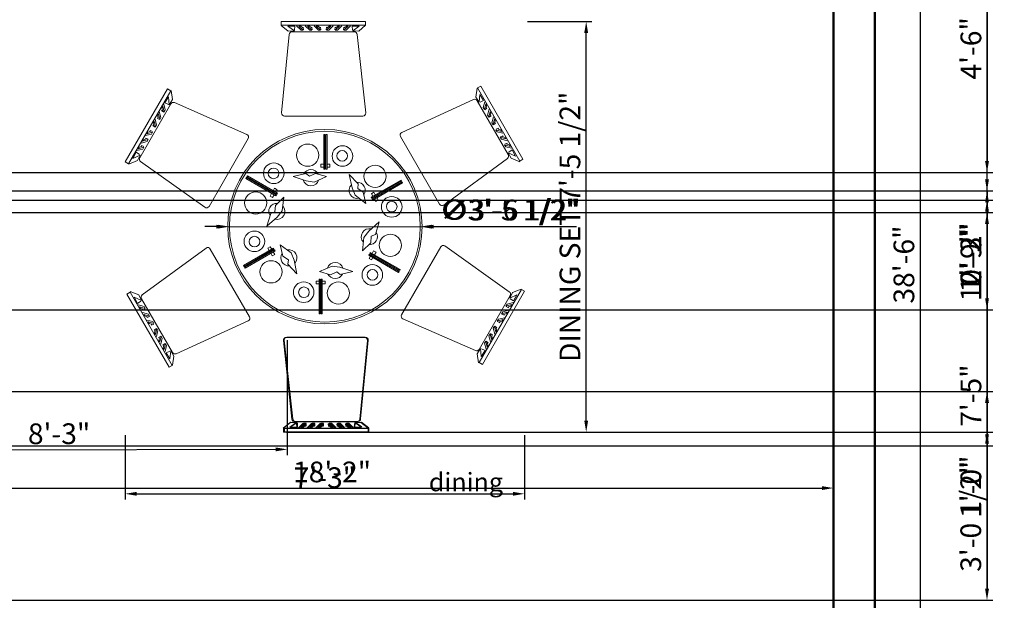
# Model space of a CAD drawing. Units: inches. Extents: x 1253 to 1645, y 2180 to 2698.
# Tile 4 of 5: x 1431 to 1645, y 2363 to 2490. Entities that reach past the tile are written whole.
import ezdxf

# ---------------------------------------------------------------- set-up
doc = ezdxf.new("R2010")
doc.units = ezdxf.units.IN
for name, color, linetype, lineweight in [('A-ANNO-DIMS', 2, 'Continuous', 18), ('A-AREA-IDEN', 7, 'Continuous', 25), ('A-FURN', 8, 'Continuous', 18), ('wall', 7, 'Continuous', 50)]:
    doc.layers.add(name, color=color, linetype=linetype, lineweight=lineweight)
doc.styles.get("Standard").update_dxf_attribs({"font": 'arial.ttf'})
doc.dimstyles.new('ISO-25', dxfattribs={"dimtxt": 4.5, "dimasz": 2.5, "dimexe": 1.25, "dimexo": 0.625, "dimtad": 1, "dimdec": 1, "dimlunit": 3, "dimtxsty": 'Standard', "dimcen": 4.5, "dimadec": 0, "dimazin": 0, "dimtfac": 1, "dimtdec": 1, "dimtmove": 0, "dimatfit": 3, "dimfxl": 1, "dimarcsym": 0})

# ---------------------------------------------------------------- blocks, each defined once
blk = doc.blocks.new('A$C45501D90')
for p, q in [((-242.2, 1133.5), (224, 1133.5)), ((-242.2, 1112.8), (-242.2, 1133.5)), ((224, 1112.8), (-242.2, 1112.8)), ((-242.2, 1111.2), (-202.3, 1079.2)), ((-203.9, 1106.4), (-165.6, 1108)), ((-168.8, 1080.8), (-203.9, 1106.4)), ((-165.6, 1108), (-167.2, 1085.6)), ((-156, 1109.6), (-132, 1085.6)), ((-119.3, 1085.6), (-143.2, 1108)), ((-143.2, 1108), (-133.6, 1108)), ((-133.6, 1108), (-122.5, 1098.4)), ((-122.5, 1098.4), (-119.3, 1101.6)), ((-119.3, 1101.6), (-117.7, 1087.2)), ((-108.1, 1109.6), (-84.1, 1085.6)), ((-71.4, 1085.6), (-95.3, 1108)), ((-95.3, 1108), (-85.7, 1108)), ((-85.7, 1108), (-74.6, 1098.4)), ((-74.6, 1098.4), (-71.4, 1101.6)), ((-71.4, 1101.6), (-69.8, 1087.2)), ((-60.2, 1109.6), (-36.2, 1085.6)), ((-23.5, 1085.6), (-47.4, 1108)), ((-47.4, 1108), (-37.8, 1108)), ((-37.8, 1108), (-26.7, 1098.4)), ((-26.7, 1098.4), (-23.5, 1101.6)), ((-23.5, 1101.6), (-21.9, 1087.2)), ((8.5, 1101.6), (6.9, 1087.2)), ((8.5, 1085.6), (32.4, 1108)), ((11.6, 1098.4), (8.5, 1101.6)), ((22.8, 1108), (11.6, 1098.4)), ((45.2, 1109.6), (21.2, 1085.6)), ((32.4, 1108), (22.8, 1108)), ((56.3, 1101.6), (54.8, 1087.2)), ((56.3, 1085.6), (80.3, 1108)), ((59.5, 1098.4), (56.3, 1101.6)), ((70.7, 1108), (59.5, 1098.4)), ((93.1, 1109.6), (69.1, 1085.6)), ((80.3, 1108), (70.7, 1108)), ((104.2, 1101.6), (102.6, 1087.2)), ((104.2, 1085.6), (128.2, 1108)), ((107.4, 1098.4), (104.2, 1101.6)), ((118.6, 1108), (107.4, 1098.4)), ((141, 1109.6), (117, 1085.6)), ((128.2, 1108), (118.6, 1108)), ((188.9, 1106.4), (150.5, 1108)), ((150.5, 1108), (152.1, 1085.6)), ((153.7, 1080.8), (188.9, 1106.4)), ((224, 1112.8), (187.3, 1079.2)), ((224, 1133.5), (224, 1112.8)), ((-197.3, 1061.6), (-238.9, 627.6)), ((-202.3, 1079.2), (-168.8, 1080.8)), ((161.8, 1076.1), (-181.4, 1076.1)), ((-132, 1085.6), (-119.3, 1085.6)), ((-84.1, 1085.6), (-71.4, 1085.6)), ((-36.2, 1085.6), (-23.5, 1085.6)), ((21.2, 1085.6), (8.5, 1085.6)), ((69.1, 1085.6), (56.3, 1085.6)), ((117, 1085.6), (104.2, 1085.6)), ((187.3, 1079.2), (153.7, 1080.8)), ((225.2, 627.8), (177.6, 1061.8)), ((841.2, 765.3), (833.5, 714.8)), ((842.6, 766.1), (860.5, 776.5)), ((1075.7, 362.4), (842.6, 766.1)), ((860.5, 776.5), (1093.6, 372.8)), ((-1102.7, 357), (-869.7, 760.7)), ((-851.7, 750.4), (-1084.8, 346.6)), ((-863.7, 716.7), (-884.3, 684.4)), ((-869.7, 760.7), (-851.7, 750.4)), ((-859.2, 673.6), (-863.7, 716.7)), ((-848.7, 752.3), (-841, 701.8)), ((833.5, 714.8), (851.7, 686.6)), ((851.7, 686.6), (856.2, 729.8)), ((856.2, 729.8), (876.7, 697.4)), ((-851, 678.1), (-1022.6, 380.9)), ((-895.4, 665), (-900.2, 656.7)), ((-900.2, 656.7), (-897.5, 642.2)), ((-888.1, 633.1), (-895.4, 665)), ((-890.4, 676.9), (-881.7, 644.2)), ((-884.3, 684.4), (-864.1, 674.6)), ((-841, 701.8), (-859.2, 673.6)), ((-431.1, 509), (-830.8, 684.8)), ((820.7, 701.7), (424.1, 520.7)), ((1012.8, 397.9), (841.2, 695.1)), ((876.7, 697.4), (856.6, 687.6)), ((882.9, 689.9), (874.2, 657.2)), ((874.2, 657.2), (880.6, 646.1)), ((880.6, 646.1), (887.9, 678)), ((894.4, 654.1), (882.7, 645.5)), ((887.9, 678), (892.7, 669.7)), ((892.7, 669.7), (890, 655.2)), ((890, 655.2), (894.4, 654.1)), ((-921.5, 600.8), (-925.8, 599.6)), ((-925.8, 599.6), (-914.2, 591)), ((-919.4, 623.5), (-924.2, 615.2)), ((-924.2, 615.2), (-921.5, 600.8)), ((-912, 591.6), (-919.4, 623.5)), ((-914.4, 635.4), (-905.6, 602.7)), ((-905.6, 602.7), (-912, 591.6)), ((-897.5, 642.2), (-901.9, 641.1)), ((-901.9, 641.1), (-890.2, 632.5)), ((-881.7, 644.2), (-888.1, 633.1)), ((-223, 610.1), (209.4, 610.1)), ((906.9, 648.4), (898.1, 615.7)), ((898.1, 615.7), (904.5, 604.6)), ((904.5, 604.6), (911.9, 636.5)), ((918.3, 612.6), (906.7, 604)), ((911.9, 636.5), (916.7, 628.2)), ((916.7, 628.2), (914, 613.8)), ((914, 613.8), (918.3, 612.6)), ((930.8, 606.9), (922.1, 574.2)), ((-945.4, 559.3), (-949.8, 558.1)), ((-949.8, 558.1), (-938.1, 549.6)), ((-943.3, 582), (-948.1, 573.8)), ((-948.1, 573.8), (-945.4, 559.3)), ((-936, 550.1), (-943.3, 582)), ((-938.3, 593.9), (-929.6, 561.2)), ((-929.6, 561.2), (-936, 550.1)), ((922.1, 574.2), (928.4, 563.1)), ((928.4, 563.1), (935.8, 595.1)), ((942.3, 571.1), (930.6, 562.6)), ((935.8, 595.1), (940.6, 586.8)), ((940.6, 586.8), (937.9, 572.3)), ((937.9, 572.3), (942.3, 571.1)), ((-991, 502.7), (-958.3, 511.4)), ((-951.9, 522.5), (-983.2, 512.9)), ((-983.2, 512.9), (-978.5, 521.2)), ((-978.5, 521.2), (-964.6, 526.1)), ((-964.6, 526.1), (-965.7, 530.5)), ((-965.7, 530.5), (-952.5, 524.7)), ((-958.3, 511.4), (-951.9, 522.5)), ((-5.6, 508.7, 90.8), (0.4, 508.7, 90.8)), ((-5.6, 317.7, 90.8), (-5.6, 508.7, 90.8)), ((0.4, 508.7, 90.8), (0.4, 317.7, 90.8)), ((5.8, 317.7, 90.8), (5.8, 508.7, 90.8)), ((5.8, 508.7, 90.8), (11.8, 508.7, 90.8)), ((11.8, 508.7, 90.8), (11.8, 317.7, 90.8)), ((416.9, 498.2), (633.1, 123.7)), ((950.8, 524.4), (944.4, 535.5)), ((944.4, 535.5), (975.7, 525.9)), ((958.2, 543.5), (945, 537.7)), ((983.5, 515.7), (950.8, 524.4)), ((957.1, 539.1), (958.2, 543.5)), ((970.9, 534.2), (957.1, 539.1)), ((968.4, 494), (999.7, 484.4)), ((974.7, 483), (968.4, 494)), ((982.2, 502), (968.9, 496.2)), ((975.7, 525.9), (970.9, 534.2)), ((981, 497.6), (982.2, 502)), ((994.9, 492.7), (981, 497.6)), ((999.7, 484.4), (994.9, 492.7)), ((-999.8, 439.5), (-1031.1, 430)), ((-1031.1, 430), (-1026.3, 438.3)), ((-1026.3, 438.3), (-1012.5, 443.1)), ((-1015, 461.2), (-982.3, 469.9)), ((-1012.5, 443.1), (-1013.6, 447.5)), ((-1013.6, 447.5), (-1000.4, 441.7)), ((-975.9, 481), (-1007.2, 471.4)), ((-1007.2, 471.4), (-1002.4, 479.7)), ((-1006.2, 428.5), (-999.8, 439.5)), ((-1002.4, 479.7), (-988.5, 484.6)), ((-988.5, 484.6), (-989.7, 489)), ((-989.7, 489), (-976.5, 483.2)), ((-982.3, 469.9), (-975.9, 481)), ((-639.9, 111.9), (-423.7, 486.4)), ((1007.4, 474.2), (974.7, 483)), ((998.7, 441.5), (992.3, 452.5)), ((992.3, 452.5), (1023.6, 443)), ((1006.1, 460.5), (992.9, 454.7)), ((1031.4, 432.7), (998.7, 441.5)), ((1005, 456.2), (1006.1, 460.5)), ((1018.8, 451.3), (1005, 456.2)), ((1023.6, 443), (1018.8, 451.3)), ((-1060.1, 376.6), (-1042.3, 410.6)), ((-1020.4, 394.3), (-1060.1, 376.6)), ((-1042.3, 410.6), (-1023.8, 398.1)), ((-1038.9, 419.7), (-1006.2, 428.5)), ((-1035.8, 364.4), (-1020.4, 394.3)), ((1028.3, 377.5), (1012.9, 407.3)), ((1012.9, 407.3), (1052.6, 389.6)), ((1034.8, 423.6), (1016.3, 411.1)), ((1052.6, 389.6), (1034.8, 423.6)), ((-1084.8, 346.6), (-1102.7, 357)), ((-1083.4, 345.8), (-1035.8, 364.4)), ((-1018, 360), (-663, 106.9)), ((-22.3, 329.1, 90.8), (-22.3, 344.6, 90.8)), ((-22.3, 344.6, 90.8), (-5.6, 344.6, 90.8)), ((-5.6, 329.1, 90.8), (-22.3, 329.1, 90.8)), ((0.4, 344.6, 90.8), (5.8, 344.6, 90.8)), ((5.8, 329.1, 90.8), (0.4, 329.1, 90.8)), ((11.8, 344.6, 90.8), (27.3, 344.6, 90.8)), ((27.3, 329.1, 90.8), (11.8, 329.1, 90.8)), ((27.3, 344.6, 90.8), (27.3, 329.1, 90.8)), ((656.3, 118.9), (1008.4, 377.1)), ((1075.9, 358.8), (1028.3, 377.5)), ((1093.6, 372.8), (1075.7, 362.4)), ((-430.6, 275.2, 90.8), (-427.6, 280.3, 90.8)), ((-265.2, 179.7, 90.8), (-430.6, 275.2, 90.8)), ((-427.6, 280.3, 90.8), (-262.3, 184.9, 90.8)), ((-175.3, 276.1, 90.8), (-104.8, 293.2, 90.8)), ((-103.3, 252.4, 90.8), (-175.3, 276.1, 90.8)), ((-104.8, 293.2, 90.8), (-85.5, 278.4, 90.8)), ((-85.5, 278.4, 90.8), (-52.1, 293.9, 90.8)), ((9.5, 276.1, 90.8), (-59.5, 246.5, 90.8)), ((-52.1, 293.9, 90.8), (9.5, 276.1, 90.8)), ((0.4, 317.7, 90.8), (-5.6, 317.7, 90.8)), ((11.8, 317.7, 90.8), (5.8, 317.7, 90.8)), ((134.3, 288, 90.8), (184.3, 235.5, 90.8)), ((149.7, 213.9, 90.8), (134.3, 288, 90.8)), ((-436.3, 265.3, 90.8), (-433.3, 270.5, 90.8)), ((-270.9, 169.9, 90.8), (-436.3, 265.3, 90.8)), ((-433.3, 270.5, 90.8), (-267.9, 175, 90.8)), ((-59.5, 246.5, 90.8), (-103.3, 252.4, 90.8)), ((184.3, 235.5, 90.8), (181.1, 211.4, 90.8)), ((255.2, 161.9, 90.8), (420.6, 257.3, 90.8)), ((423.5, 252.2, 90.8), (258.2, 156.7, 90.8)), ((260.9, 152, 90.8), (426.2, 247.5, 90.8)), ((429.2, 242.3, 90.8), (263.8, 146.9, 90.8)), ((420.6, 257.3, 90.8), (423.5, 252.2, 90.8)), ((426.2, 247.5, 90.8), (429.2, 242.3, 90.8)), ((-302.5, 168.8, 90.8), (-294.2, 183.3, 90.8)), ((-289.1, 161.1, 90.8), (-302.5, 168.8, 90.8)), ((-291.2, 188.5, 90.8), (-288.5, 193.1, 90.8)), ((-280.7, 175.5, 90.8), (-289.1, 161.1, 90.8)), ((-285.5, 198.3, 90.8), (-277.8, 211.7, 90.8)), ((-277.8, 211.7, 90.8), (-264.3, 204, 90.8)), ((-275.1, 185.4, 90.8), (-277.8, 180.7, 90.8)), ((-264.3, 204, 90.8), (-272.1, 190.5, 90.8)), ((-267.9, 175, 90.8), (-270.9, 169.9, 90.8)), ((-262.3, 184.9, 90.8), (-265.2, 179.7, 90.8)), ((166.5, 173, 90.8), (149.7, 213.9, 90.8)), ((226.7, 128.1, 90.8), (166.5, 173, 90.8)), ((181.1, 211.4, 90.8), (211.3, 190.3, 90.8)), ((211.3, 190.3, 90.8), (226.7, 128.1, 90.8)), ((256.6, 182, 90.8), (270.1, 189.8, 90.8)), ((265, 167.5, 90.8), (256.6, 182, 90.8)), ((270.1, 189.8, 90.8), (278.4, 175.3, 90.8)), ((281.4, 170.1, 90.8), (284.1, 165.5, 90.8)), ((-276.8, 80.9, 90.8), (-273.6, 117.6, 90.8)), ((-273.6, 117.6, 90.8), (-227.4, 162.1, 90.8)), ((-227.4, 162.1, 90.8), (-236.2, 87.5, 90.8)), ((258.2, 156.7, 90.8), (255.2, 161.9, 90.8)), ((263.8, 146.9, 90.8), (260.9, 152, 90.8)), ((270.7, 157.7, 90.8), (268, 162.4, 90.8)), ((281.4, 139.1, 90.8), (273.7, 152.5, 90.8)), ((294.9, 146.8, 90.8), (281.4, 139.1, 90.8)), ((287.1, 160.3, 90.8), (294.9, 146.8, 90.8)), ((-319.8, 2.1, 90.8), (-299.3, 71.7, 90.8)), ((-299.3, 71.7, 90.8), (-276.8, 80.9, 90.8)), ((-236.2, 87.5, 90.8), (-263.2, 52.5, 90.8)), ((-263.2, 52.5, 90.8), (-319.8, 2.1, 90.8)), ((242.9, -24.6, 90.8), (299.4, 25.9, 90.8)), ((299.4, 25.9, 90.8), (278.9, -43.7, 90.8)), ((215.8, -59.5, 90.8), (242.9, -24.6, 90.8)), ((256.4, -53, 90.8), (253.2, -89.7, 90.8)), ((278.9, -43.7, 90.8), (256.4, -53, 90.8)), ((-247, -100.1, 90.8), (-186.8, -145, 90.8)), ((-231.7, -162.3, 90.8), (-247, -100.1, 90.8)), ((207, -134.1, 90.8), (215.8, -59.5, 90.8)), ((253.2, -89.7, 90.8), (207, -134.1, 90.8)), ((1018, -360), (663, -106.9)), ((-656.3, -118.9), (-1008.4, -377.1)), ((-416.9, -498.2), (-633.1, -123.7)), ((-449.6, -214.4, 90.8), (-284.2, -118.9, 90.8)), ((-281.2, -124.1, 90.8), (-446.6, -219.5, 90.8)), ((-443.9, -224.2, 90.8), (-278.5, -128.7, 90.8)), ((-275.5, -133.9, 90.8), (-440.9, -229.4, 90.8)), ((-315.2, -118.9, 90.8), (-301.8, -111.1, 90.8)), ((-307.5, -132.3, 90.8), (-315.2, -118.9, 90.8)), ((-301.8, -142.1, 90.8), (-304.5, -137.5, 90.8)), ((-301.8, -111.1, 90.8), (-294, -124.6, 90.8)), ((-290.4, -161.8, 90.8), (-298.8, -147.3, 90.8)), ((-291, -129.7, 90.8), (-288.3, -134.4, 90.8)), ((-277, -154, 90.8), (-290.4, -161.8, 90.8)), ((-285.4, -139.5, 90.8), (-277, -154, 90.8)), ((-284.2, -118.9, 90.8), (-281.2, -124.1, 90.8)), ((-278.5, -128.7, 90.8), (-275.5, -133.9, 90.8)), ((-201.5, -183.4, 90.8), (-231.7, -162.3, 90.8)), ((-186.8, -145, 90.8), (-170.1, -185.9, 90.8)), ((241.9, -156.9, 90.8), (244.9, -151.7, 90.8)), ((407.3, -252.4, 90.8), (241.9, -156.9, 90.8)), ((244, -176, 90.8), (251.7, -162.5, 90.8)), ((244.9, -151.7, 90.8), (410.3, -247.2, 90.8)), ((247.6, -147.1, 90.8), (250.6, -141.9, 90.8)), ((413, -242.5, 90.8), (247.6, -147.1, 90.8)), ((250.6, -141.9, 90.8), (415.9, -237.4, 90.8)), ((254.7, -157.4, 90.8), (257.4, -152.7, 90.8)), ((260.4, -147.6, 90.8), (268.7, -133.1, 90.8)), ((270.8, -160.5, 90.8), (268.1, -165.1, 90.8)), ((268.7, -133.1, 90.8), (282.2, -140.8, 90.8)), ((282.2, -140.8, 90.8), (273.8, -155.3, 90.8)), ((639.9, -111.9), (423.7, -486.4)), ((-446.6, -219.5, 90.8), (-449.6, -214.4, 90.8)), ((-204.7, -207.6, 90.8), (-201.5, -183.4, 90.8)), ((-154.7, -260.1, 90.8), (-204.7, -207.6, 90.8)), ((-170.1, -185.9, 90.8), (-154.7, -260.1, 90.8)), ((257.4, -183.7, 90.8), (244, -176, 90.8)), ((265.2, -170.3, 90.8), (257.4, -183.7, 90.8)), ((-440.9, -229.4, 90.8), (-443.9, -224.2, 90.8)), ((-29.8, -248.2, 90.8), (39.2, -218.5, 90.8)), ((31.8, -266, 90.8), (-29.8, -248.2, 90.8)), ((65.2, -250.4, 90.8), (31.8, -266, 90.8)), ((39.2, -218.5, 90.8), (83, -224.4, 90.8)), ((84.4, -265.2, 90.8), (65.2, -250.4, 90.8)), ((83, -224.4, 90.8), (154.9, -248.2, 90.8)), ((154.9, -248.2, 90.8), (84.4, -265.2, 90.8)), ((410.3, -247.2, 90.8), (407.3, -252.4, 90.8)), ((415.9, -237.4, 90.8), (413, -242.5, 90.8)), ((-47.6, -316.6, 90.8), (-47.6, -301.1, 90.8)), ((-47.6, -301.1, 90.8), (-32.1, -301.1, 90.8)), ((-32.1, -316.6, 90.8), (-47.6, -316.6, 90.8)), ((-32.1, -480.7, 90.8), (-32.1, -289.8, 90.8)), ((-32.1, -289.8, 90.8), (-26.1, -289.8, 90.8)), ((-26.1, -289.8, 90.8), (-26.1, -480.7, 90.8)), ((-26.1, -301.1, 90.8), (-20.8, -301.1, 90.8)), ((-20.8, -316.6, 90.8), (-26.1, -316.6, 90.8)), ((-20.8, -480.7, 90.8), (-20.8, -289.8, 90.8)), ((-20.8, -289.8, 90.8), (-14.8, -289.8, 90.8)), ((-14.8, -289.8, 90.8), (-14.8, -480.7, 90.8)), ((-14.8, -301.1, 90.8), (1.9, -301.1, 90.8)), ((1.9, -316.6, 90.8), (-14.8, -316.6, 90.8)), ((1.9, -301.1, 90.8), (1.9, -316.6, 90.8)), ((-1093.6, -372.8), (-1075.7, -362.4)), ((-860.5, -776.5), (-1093.6, -372.8)), ((-1075.9, -358.8), (-1028.3, -377.5)), ((-1075.7, -362.4), (-842.6, -766.1)), ((-1028.3, -377.5), (-1012.9, -407.3)), ((851.7, -750.4), (1084.8, -346.6)), ((1102.7, -357), (869.7, -760.7)), ((1035.8, -364.4), (1020.4, -394.3)), ((1020.4, -394.3), (1060.1, -376.6)), ((1083.4, -345.8), (1035.8, -364.4)), ((1060.1, -376.6), (1042.3, -410.6)), ((1084.8, -346.6), (1102.7, -357)), ((-1052.6, -389.6), (-1034.8, -423.6)), ((-1012.9, -407.3), (-1052.6, -389.6)), ((-1034.8, -423.6), (-1016.3, -411.1)), ((-1031.4, -432.7), (-998.7, -441.5)), ((-1012.8, -397.9), (-841.2, -695.1)), ((851, -678.1), (1022.6, -380.9)), ((1006.2, -428.5), (999.8, -439.5)), ((999.8, -439.5), (1031.1, -430)), ((1038.9, -419.7), (1006.2, -428.5)), ((1042.3, -410.6), (1023.8, -398.1)), ((1031.1, -430), (1026.3, -438.3)), ((-1023.6, -443), (-1018.8, -451.3)), ((-992.3, -452.5), (-1023.6, -443)), ((-1018.8, -451.3), (-1005, -456.2)), ((-1007.4, -474.2), (-974.7, -483)), ((-1006.1, -460.5), (-992.9, -454.7)), ((-1005, -456.2), (-1006.1, -460.5)), ((-968.4, -494), (-999.7, -484.4)), ((-999.7, -484.4), (-994.9, -492.7)), ((-998.7, -441.5), (-992.3, -452.5)), ((-974.7, -483), (-968.4, -494)), ((-26.1, -480.7, 90.8), (-32.1, -480.7, 90.8)), ((-14.8, -480.7, 90.8), (-20.8, -480.7, 90.8)), ((982.3, -469.9), (975.9, -481)), ((975.9, -481), (1007.2, -471.4)), ((989.7, -489), (976.5, -483.2)), ((1015, -461.2), (982.3, -469.9)), ((1002.4, -479.7), (988.5, -484.6)), ((988.5, -484.6), (989.7, -489)), ((1013.6, -447.5), (1000.4, -441.7)), ((1007.2, -471.4), (1002.4, -479.7)), ((1026.3, -438.3), (1012.5, -443.1)), ((1012.5, -443.1), (1013.6, -447.5)), ((-994.9, -492.7), (-981, -497.6)), ((-983.5, -515.7), (-950.8, -524.4)), ((-982.2, -502), (-968.9, -496.2)), ((-981, -497.6), (-982.2, -502)), ((-944.4, -535.5), (-975.7, -525.9)), ((-975.7, -525.9), (-970.9, -534.2)), ((-970.9, -534.2), (-957.1, -539.1)), ((-958.2, -543.5), (-945, -537.7)), ((-957.1, -539.1), (-958.2, -543.5)), ((-950.8, -524.4), (-944.4, -535.5)), ((-820.7, -701.7), (-424.1, -520.7)), ((431.1, -509), (830.8, -684.8)), ((958.3, -511.4), (951.9, -522.5)), ((951.9, -522.5), (983.2, -512.9)), ((965.7, -530.5), (952.5, -524.7)), ((991, -502.7), (958.3, -511.4)), ((978.5, -521.2), (964.6, -526.1)), ((964.6, -526.1), (965.7, -530.5)), ((983.2, -512.9), (978.5, -521.2)), ((-942.3, -571.1), (-930.6, -562.6)), ((-937.9, -572.3), (-942.3, -571.1)), ((-940.6, -586.8), (-937.9, -572.3)), ((-935.8, -595.1), (-940.6, -586.8)), ((-928.4, -563.1), (-935.8, -595.1)), ((-930.8, -606.9), (-922.1, -574.2)), ((-922.1, -574.2), (-928.4, -563.1)), ((905.6, -602.7), (912, -591.6)), ((912, -591.6), (919.4, -623.5)), ((925.8, -599.6), (914.2, -591)), ((929.6, -561.2), (936, -550.1)), ((938.3, -593.9), (929.6, -561.2)), ((936, -550.1), (943.3, -582)), ((949.8, -558.1), (938.1, -549.6)), ((943.3, -582), (948.1, -573.8)), ((945.4, -559.3), (949.8, -558.1)), ((948.1, -573.8), (945.4, -559.3)), ((-918.3, -612.6), (-906.7, -604)), ((-914, -613.8), (-918.3, -612.6)), ((-916.7, -628.2), (-914, -613.8)), ((-911.9, -636.5), (-916.7, -628.2)), ((-904.5, -604.6), (-911.9, -636.5)), ((-906.9, -648.4), (-898.1, -615.7)), ((-898.1, -615.7), (-904.5, -604.6)), ((-894.4, -654.1), (-882.7, -645.5)), ((-880.6, -646.1), (-887.9, -678)), ((-874.2, -657.2), (-880.6, -646.1)), ((-229.3, -629.3), (-181.8, -1063.3)), ((-225.2, -627.8), (-177.6, -1061.8)), ((218.9, -611.6), (-213.5, -611.6)), ((223, -610.1), (-209.4, -610.1)), ((193.2, -1063.1), (234.8, -629.1)), ((197.3, -1061.6), (238.9, -627.6)), ((881.7, -644.2), (888.1, -633.1)), ((890.4, -676.9), (881.7, -644.2)), ((888.1, -633.1), (895.4, -665)), ((901.9, -641.1), (890.2, -632.5)), ((897.5, -642.2), (901.9, -641.1)), ((900.2, -656.7), (897.5, -642.2)), ((914.4, -635.4), (905.6, -602.7)), ((919.4, -623.5), (924.2, -615.2)), ((921.5, -600.8), (925.8, -599.6)), ((924.2, -615.2), (921.5, -600.8)), ((-890, -655.2), (-894.4, -654.1)), ((-892.7, -669.7), (-890, -655.2)), ((-887.9, -678), (-892.7, -669.7)), ((-882.9, -689.9), (-874.2, -657.2)), ((-876.7, -697.4), (-856.6, -687.6)), ((-856.2, -729.8), (-876.7, -697.4)), ((-851.7, -686.6), (-856.2, -729.8)), ((-833.5, -714.8), (-851.7, -686.6)), ((841, -701.8), (859.2, -673.6)), ((848.7, -752.3), (841, -701.8)), ((859.2, -673.6), (863.7, -716.7)), ((863.7, -716.7), (884.3, -684.4)), ((884.3, -684.4), (864.1, -674.6)), ((895.4, -665), (900.2, -656.7)), ((-841.2, -765.3), (-833.5, -714.8)), ((869.7, -760.7), (851.7, -750.4)), ((-842.6, -766.1), (-860.5, -776.5)), ((-231.3, -1112.7), (-191.4, -1080.8)), ((-227.2, -1111.2), (-187.3, -1079.2)), ((-157.9, -1082.4), (-193, -1107.9)), ((-191.4, -1080.8), (-157.9, -1082.4)), ((-153.7, -1080.8), (-188.9, -1106.4)), ((-187.3, -1079.2), (-153.7, -1080.8)), ((-165.9, -1077.6), (177.3, -1077.6)), ((-161.8, -1076.1), (181.4, -1076.1)), ((-154.7, -1109.5), (-156.3, -1087.1)), ((-150.5, -1108), (-152.1, -1085.6)), ((-145.1, -1111.1), (-121.1, -1087.1)), ((-141, -1109.6), (-117, -1085.6)), ((-108.4, -1087.1), (-132.3, -1109.5)), ((-104.2, -1085.6), (-128.2, -1108)), ((-121.1, -1087.1), (-108.4, -1087.1)), ((-117, -1085.6), (-104.2, -1085.6)), ((-104.2, -1101.6), (-102.6, -1087.2)), ((-97.2, -1111.1), (-73.2, -1087.1)), ((-93.1, -1109.6), (-69.1, -1085.6)), ((-60.5, -1087.1), (-84.4, -1109.5)), ((-56.3, -1085.6), (-80.3, -1108)), ((-73.2, -1087.1), (-60.5, -1087.1)), ((-69.1, -1085.6), (-56.3, -1085.6)), ((-56.3, -1101.6), (-54.8, -1087.2)), ((-49.3, -1111.1), (-25.3, -1087.1)), ((-45.2, -1109.6), (-21.2, -1085.6)), ((-12.6, -1087.1), (-36.5, -1109.5)), ((-8.5, -1085.6), (-32.4, -1108)), ((-25.3, -1087.1), (-12.6, -1087.1)), ((-21.2, -1085.6), (-8.5, -1085.6)), ((-8.5, -1101.6), (-6.9, -1087.2)), ((19.4, -1087.1), (43.3, -1109.5)), ((32.1, -1087.1), (19.4, -1087.1)), ((23.5, -1101.6), (21.9, -1087.2)), ((23.5, -1085.6), (47.4, -1108)), ((36.2, -1085.6), (23.5, -1085.6)), ((56.1, -1111.1), (32.1, -1087.1)), ((60.2, -1109.6), (36.2, -1085.6)), ((67.3, -1087.1), (91.2, -1109.5)), ((80, -1087.1), (67.3, -1087.1)), ((71.4, -1101.6), (69.8, -1087.2)), ((71.4, -1085.6), (95.3, -1108)), ((84.1, -1085.6), (71.4, -1085.6)), ((104, -1111.1), (80, -1087.1)), ((108.1, -1109.6), (84.1, -1085.6)), ((115.1, -1087.1), (139.1, -1109.5)), ((127.9, -1087.1), (115.1, -1087.1)), ((119.3, -1101.6), (117.7, -1087.2)), ((119.3, -1085.6), (143.2, -1108)), ((132, -1085.6), (119.3, -1085.6)), ((151.9, -1111.1), (127.9, -1087.1)), ((156, -1109.6), (132, -1085.6)), ((161.4, -1109.5), (163, -1087.1)), ((198.2, -1080.8), (164.6, -1082.4)), ((164.6, -1082.4), (199.8, -1107.9)), ((165.6, -1108), (167.2, -1085.6)), ((202.3, -1079.2), (168.8, -1080.8)), ((168.8, -1080.8), (203.9, -1106.4)), ((238.1, -1112.7), (198.2, -1080.8)), ((242.2, -1111.2), (202.3, -1079.2)), ((-228.1, -1114.3), (238.1, -1114.3)), ((-228.1, -1135), (-228.1, -1114.3)), ((238.1, -1135), (-228.1, -1135)), ((-224, -1112.8), (242.2, -1112.8)), ((-224, -1133.5), (-224, -1112.8)), ((242.2, -1133.5), (-224, -1133.5)), ((-193, -1107.9), (-154.7, -1109.5)), ((-188.9, -1106.4), (-150.5, -1108)), ((-132.3, -1109.5), (-122.7, -1109.5)), ((-128.2, -1108), (-118.6, -1108)), ((-122.7, -1109.5), (-111.6, -1099.9)), ((-118.6, -1108), (-107.4, -1098.4)), ((-111.6, -1099.9), (-108.4, -1103.1)), ((-108.4, -1103.1), (-106.8, -1088.7)), ((-107.4, -1098.4), (-104.2, -1101.6)), ((-84.4, -1109.5), (-74.8, -1109.5)), ((-80.3, -1108), (-70.7, -1108)), ((-74.8, -1109.5), (-63.7, -1099.9)), ((-70.7, -1108), (-59.5, -1098.4)), ((-63.7, -1099.9), (-60.5, -1103.1)), ((-60.5, -1103.1), (-58.9, -1088.7)), ((-59.5, -1098.4), (-56.3, -1101.6)), ((-36.5, -1109.5), (-26.9, -1109.5)), ((-32.4, -1108), (-22.8, -1108)), ((-26.9, -1109.5), (-15.8, -1099.9)), ((-22.8, -1108), (-11.6, -1098.4)), ((-15.8, -1099.9), (-12.6, -1103.1)), ((-12.6, -1103.1), (-11, -1088.7)), ((-11.6, -1098.4), (-8.5, -1101.6)), ((19.4, -1103.1), (17.8, -1088.7)), ((22.6, -1099.9), (19.4, -1103.1)), ((33.7, -1109.5), (22.6, -1099.9)), ((26.7, -1098.4), (23.5, -1101.6)), ((37.8, -1108), (26.7, -1098.4)), ((43.3, -1109.5), (33.7, -1109.5)), ((47.4, -1108), (37.8, -1108)), ((67.3, -1103.1), (65.7, -1088.7)), ((70.4, -1099.9), (67.3, -1103.1)), ((81.6, -1109.5), (70.4, -1099.9)), ((74.6, -1098.4), (71.4, -1101.6)), ((85.7, -1108), (74.6, -1098.4)), ((91.2, -1109.5), (81.6, -1109.5)), ((95.3, -1108), (85.7, -1108)), ((115.1, -1103.1), (113.6, -1088.7)), ((118.3, -1099.9), (115.1, -1103.1)), ((129.5, -1109.5), (118.3, -1099.9)), ((122.5, -1098.4), (119.3, -1101.6)), ((133.6, -1108), (122.5, -1098.4)), ((139.1, -1109.5), (129.5, -1109.5)), ((143.2, -1108), (133.6, -1108)), ((199.8, -1107.9), (161.4, -1109.5)), ((203.9, -1106.4), (165.6, -1108)), ((238.1, -1114.3), (238.1, -1135)), ((242.2, -1112.8), (242.2, -1133.5))]:
    blk.add_line(p, q)
for centre, radius in [((0, 0), 537), ((0, 0), 527), ((-94.8, 394.7, 90.8), 61.3), ((96.9, 390, 90.8), 56.9), ((95.5, 390.7, 90.8), 29.4), ((-282.3, 294.7, 90.8), 56.9), ((277.2, 277.6, 90.8), 61.3), ((-283.5, 293.9, 90.8), 29.4), ((-382.1, 131.1, 90.8), 61.3), ((369, 109.3, 90.8), 56.9), ((368.9, 110.8, 90.8), 29.4), ((-389.3, -81.3, 90.8), 56.9), ((-389.2, -82.8, 90.8), 29.4), ((361.8, -103.1, 90.8), 61.3), ((-297.5, -249.6, 90.8), 61.3), ((261.9, -266.7, 90.8), 56.9), ((263.2, -265.9, 90.8), 29.4), ((-117.2, -362, 90.8), 56.9), ((74.4, -366.7, 90.8), 61.3), ((-115.9, -362.7, 90.8), 29.4)]:
    blk.add_circle(centre, radius)
for centre, radius, start, end in [((-181.4, 1060.1), 16, 90, 174.5199), ((161.8, 1060.1), 16, 6.2572, 90), ((-837.2, 670.1), 16, 66.2572, 150), ((827.4, 687.1), 16, 30, 114.5199), ((-223, 626.1), 16, 174.5199, 270), ((209.4, 626.1), 16, 270, 6.2572), ((-437.5, 494.4), 16, 330, 66.2572), ((430.7, 506.2), 16, 114.5199, 210), ((-1008.8, 373), 16, 150, 234.5199), ((999, 389.9), 16, 306.2572, 30), ((-77.3, 270.2, 90.8), 44.6, 25.8558, 153.3359), ((-77.3, 270.2, 90.8), 44.6, 195.9338, 342.9389), ((178.1, 200.3, 90.8), 44.6, 135.9338, 282.9389), ((178.1, 200.3, 90.8), 44.6, 325.8558, 93.3359), ((-653.7, 119.9), 16, 234.5199, 330), ((-265.7, 83.9, 90.8), 44.6, 85.8558, 213.3359), ((-265.7, 83.9, 90.8), 44.6, 255.9338, 42.9389), ((646.9, 131.7), 16, 210, 306.2572), ((245.3, -55.9, 90.8), 44.6, 75.9338, 222.9389), ((245.3, -55.9, 90.8), 44.6, 265.8558, 33.3359), ((653.7, -119.9), 16, 54.5199, 150), ((-646.9, -131.7), 16, 30, 126.2572), ((-198.5, -172.3, 90.8), 44.6, 145.8558, 273.3359), ((-198.5, -172.3, 90.8), 44.6, 315.9338, 102.9389), ((57, -242.2, 90.8), 44.6, 15.9338, 162.9389), ((57, -242.2, 90.8), 44.6, 205.8558, 333.3359), ((-999, -389.9), 16, 126.2572, 210), ((1008.8, -373), 16, 330, 54.5199), ((437.5, -494.4), 16, 150, 246.2572), ((-430.7, -506.2), 16, 294.5199, 30), ((-213.5, -627.6), 16, 90, 186.2572), ((-209.4, -626.1), 16, 90, 186.2572), ((218.9, -627.6), 16, 354.5199, 90), ((223, -626.1), 16, 354.5199, 90), ((-827.4, -687.1), 16, 210, 294.5199), ((837.2, -670.1), 16, 246.2572, 330), ((-165.9, -1061.6), 16, 186.2572, 270), ((-161.8, -1060.1), 16, 186.2572, 270), ((177.3, -1061.6), 16, 270, 354.5199), ((181.4, -1060.1), 16, 270, 354.5199)]:
    blk.add_arc(centre, radius, start, end)
blk = doc.blocks.new('*D14')
at = {"layer": 'A-ANNO-DIMS', "color": 0, "lineweight": -2, "transparency": 16777216}
for p, q in [((1617.57, 2667.35), (1628.02, 2667.35)), ((1626.77, 2664.85), (1626.77, 2207.85)), ((1617.57, 2205.35), (1628.02, 2205.35))]:
    blk.add_line(p, q, dxfattribs=at)
at = {"layer": 'A-ANNO-DIMS', "color": 0, "transparency": 16777216}
for points in [[(1626.36, 2664.85), (1627.19, 2664.85), (1626.77, 2667.35)], [(1626.36, 2207.85), (1627.19, 2207.85), (1626.77, 2205.35)]]:
    blk.add_solid(points, dxfattribs=at)
at = {"layer": 'Defpoints', "color": 0, "transparency": 16777216}
for p in [(1616.94, 2667.35), (1616.94, 2205.35), (1626.77, 2205.35)]:
    blk.add_point(p, dxfattribs=at)
at = {"layer": 'A-ANNO-DIMS', "color": 0, "transparency": 16777216, "insert": (1623.85, 2436.35), "char_height": 4.5, "attachment_point": 5, "rotation": 90}
blk.add_mtext('38\'-6"', dxfattribs=at)
blk = doc.blocks.new('*D26')
at = {"layer": 'A-ANNO-DIMS', "color": 0, "lineweight": -2, "transparency": 16777216}
for p, q in [((1541.42, 2489.21), (1555.44, 2489.21)), ((1554.19, 2402.4), (1554.19, 2486.71)), ((1541.42, 2399.9), (1555.44, 2399.9))]:
    blk.add_line(p, q, dxfattribs=at)
at = {"layer": 'A-ANNO-DIMS', "color": 0, "transparency": 16777216}
for points in [[(1553.77, 2486.71), (1554.61, 2486.71), (1554.19, 2489.21)], [(1553.77, 2402.4), (1554.61, 2402.4), (1554.19, 2399.9)]]:
    blk.add_solid(points, dxfattribs=at)
at = {"layer": 'Defpoints', "color": 0, "transparency": 16777216}
for p in [(1540.79, 2489.21), (1554.19, 2489.21), (1540.79, 2399.9)]:
    blk.add_point(p, dxfattribs=at)
at = {"layer": 'A-ANNO-DIMS', "color": 0, "transparency": 16777216, "insert": (1551.24, 2444.56), "char_height": 4.5, "attachment_point": 5, "rotation": 90}
blk.add_mtext('DINING SET 7\'-5 1/2"', dxfattribs=at)
blk = doc.blocks.new('*D27')
at = {"layer": 'A-ANNO-DIMS', "color": 0, "lineweight": -2, "transparency": 16777216}
for p, q in [((1453.96, 2399.27), (1453.96, 2385.25)), ((1540.79, 2399.27), (1540.79, 2385.25)), ((1456.46, 2386.5), (1538.29, 2386.5))]:
    blk.add_line(p, q, dxfattribs=at)
at = {"layer": 'A-ANNO-DIMS', "color": 0, "transparency": 16777216}
for points in [[(1456.46, 2386.92), (1456.46, 2386.09), (1453.96, 2386.5)], [(1538.29, 2386.92), (1538.29, 2386.09), (1540.79, 2386.5)]]:
    blk.add_solid(points, dxfattribs=at)
at = {"layer": 'Defpoints', "color": 0, "transparency": 16777216}
for p in [(1453.96, 2399.9), (1540.79, 2399.9), (1540.79, 2386.5)]:
    blk.add_point(p, dxfattribs=at)
at = {"layer": 'A-ANNO-DIMS', "color": 0, "transparency": 16777216, "insert": (1497.38, 2389.43), "char_height": 4.5, "attachment_point": 5}
blk.add_mtext('7\'-3"', dxfattribs=at)
blk = doc.blocks.new('*D31')
at = {"layer": 'A-ANNO-DIMS', "color": 0, "lineweight": -2, "transparency": 16777216}
for p, q in [((1386.57, 2510.35), (1642.59, 2510.35)), ((1641.34, 2507.85), (1641.34, 2458.85)), ((1386.57, 2456.35), (1642.59, 2456.35))]:
    blk.add_line(p, q, dxfattribs=at)
at = {"layer": 'A-ANNO-DIMS', "color": 0, "transparency": 16777216}
for points in [[(1640.92, 2507.85), (1641.76, 2507.85), (1641.34, 2510.35)], [(1640.92, 2458.85), (1641.76, 2458.85), (1641.34, 2456.35)]]:
    blk.add_solid(points, dxfattribs=at)
at = {"layer": 'Defpoints', "color": 0, "transparency": 16777216}
for p in [(1385.94, 2510.35), (1385.94, 2456.35), (1641.34, 2456.35)]:
    blk.add_point(p, dxfattribs=at)
at = {"layer": 'A-ANNO-DIMS', "color": 0, "transparency": 16777216, "insert": (1638.42, 2483.35), "char_height": 4.5, "attachment_point": 5, "rotation": 90}
blk.add_mtext('4\'-6"', dxfattribs=at)
blk = doc.blocks.new('*D32')
at = {"layer": 'A-ANNO-DIMS', "color": 0, "lineweight": -2, "transparency": 16777216}
for p, q in [((1386.57, 2452.35), (1642.59, 2452.35)), ((1641.34, 2449.85), (1641.34, 2365.85)), ((1386.57, 2363.35), (1642.59, 2363.35))]:
    blk.add_line(p, q, dxfattribs=at)
at = {"layer": 'A-ANNO-DIMS', "color": 0, "transparency": 16777216}
for points in [[(1640.92, 2449.85), (1641.76, 2449.85), (1641.34, 2452.35)], [(1640.92, 2365.85), (1641.76, 2365.85), (1641.34, 2363.35)]]:
    blk.add_solid(points, dxfattribs=at)
at = {"layer": 'Defpoints', "color": 0, "transparency": 16777216}
for p in [(1385.94, 2452.35), (1385.94, 2363.35), (1641.34, 2363.35)]:
    blk.add_point(p, dxfattribs=at)
at = {"layer": 'A-ANNO-DIMS', "color": 0, "transparency": 16777216, "insert": (1638.43, 2407.85), "char_height": 4.5, "attachment_point": 5, "rotation": 90}
blk.add_mtext('7\'-5"', dxfattribs=at)
blk = doc.blocks.new('*D47')
at = {"layer": 'A-ANNO-DIMS', "color": 0, "lineweight": -2, "transparency": 16777216}
for p, q in [((1641.34, 2454.85), (1641.34, 2457.35)), ((1386.57, 2452.35), (1642.59, 2452.35)), ((1641.34, 2452.35), (1641.34, 2450.35)), ((1386.57, 2450.35), (1642.59, 2450.35)), ((1641.34, 2447.85), (1641.34, 2432.13))]:
    blk.add_line(p, q, dxfattribs=at)
at = {"layer": 'A-ANNO-DIMS', "color": 0, "transparency": 16777216}
for points in [[(1640.92, 2454.85), (1641.76, 2454.85), (1641.34, 2452.35)], [(1640.92, 2447.85), (1641.76, 2447.85), (1641.34, 2450.35)]]:
    blk.add_solid(points, dxfattribs=at)
at = {"layer": 'Defpoints', "color": 0, "transparency": 16777216}
for p in [(1385.94, 2452.35), (1385.94, 2450.35), (1641.34, 2450.35)]:
    blk.add_point(p, dxfattribs=at)
at = {"layer": 'A-ANNO-DIMS', "color": 0, "transparency": 16777216, "insert": (1638.42, 2438.74), "char_height": 4.5, "attachment_point": 5, "rotation": 90}
blk.add_mtext('0\'-2"', dxfattribs=at)
blk = doc.blocks.new('*D50')
at = {"layer": 'A-ANNO-DIMS', "color": 0, "lineweight": -2, "transparency": 16777216}
for p, q in [((1363.3, 2408.78), (1642.59, 2408.78)), ((1641.34, 2406.28), (1641.34, 2399.44)), ((1363.3, 2396.94), (1642.59, 2396.94)), ((1641.34, 2396.94), (1641.34, 2381.65))]:
    blk.add_line(p, q, dxfattribs=at)
at = {"layer": 'A-ANNO-DIMS', "color": 0, "transparency": 16777216}
for points in [[(1640.92, 2406.28), (1641.76, 2406.28), (1641.34, 2408.78)], [(1640.92, 2399.44), (1641.76, 2399.44), (1641.34, 2396.94)]]:
    blk.add_solid(points, dxfattribs=at)
at = {"layer": 'Defpoints', "color": 0, "transparency": 16777216}
for p in [(1362.68, 2408.78), (1362.68, 2396.94), (1641.34, 2396.94)]:
    blk.add_point(p, dxfattribs=at)
at = {"layer": 'A-ANNO-DIMS', "color": 0, "transparency": 16777216, "insert": (1638.42, 2388.04), "char_height": 4.5, "attachment_point": 5, "rotation": 90}
blk.add_mtext('1\'-0"', dxfattribs=at)
blk = doc.blocks.new('*D55')
at = {"layer": 'A-ANNO-DIMS', "color": 0, "lineweight": -2, "transparency": 16777216}
for p, q in [((1304.46, 2447.68), (1642.59, 2447.68)), ((1641.34, 2445.18), (1641.34, 2429)), ((1304.46, 2426.5), (1642.59, 2426.5))]:
    blk.add_line(p, q, dxfattribs=at)
at = {"layer": 'A-ANNO-DIMS', "color": 0, "transparency": 16777216}
for points in [[(1640.92, 2445.18), (1641.76, 2445.18), (1641.34, 2447.68)], [(1640.92, 2429), (1641.76, 2429), (1641.34, 2426.5)]]:
    blk.add_solid(points, dxfattribs=at)
at = {"layer": 'Defpoints', "color": 0, "transparency": 16777216}
for p in [(1303.84, 2447.68), (1303.84, 2426.5), (1641.34, 2426.5)]:
    blk.add_point(p, dxfattribs=at)
at = {"layer": 'A-ANNO-DIMS', "color": 0, "transparency": 16777216, "insert": (1638.42, 2437.09), "char_height": 4.5, "attachment_point": 5, "rotation": 90}
blk.add_mtext('1\'-9"', dxfattribs=at)
blk = doc.blocks.new('*D56')
at = {"layer": 'A-ANNO-DIMS', "color": 0, "lineweight": -2, "transparency": 16777216}
for p, q in [((1389.94, 2419.72), (1390, 2394.7)), ((1489.14, 2419.94), (1489.19, 2394.91)), ((1486.69, 2396.16), (1392.5, 2395.95))]:
    blk.add_line(p, q, dxfattribs=at)
at = {"layer": 'A-ANNO-DIMS', "color": 0, "transparency": 16777216}
for points in [[(1392.49, 2396.37), (1392.5, 2395.54), (1390, 2395.95)], [(1486.69, 2396.58), (1486.69, 2395.74), (1489.19, 2396.16)]]:
    blk.add_solid(points, dxfattribs=at)
at = {"layer": 'Defpoints', "color": 0, "transparency": 16777216}
for p in [(1389.94, 2420.35), (1489.14, 2420.56), (1390, 2395.95)]:
    blk.add_point(p, dxfattribs=at)
at = {"layer": 'A-ANNO-DIMS', "color": 0, "transparency": 16777216, "insert": (1439.59, 2398.98), "char_height": 4.5, "attachment_point": 5, "rotation": 0.126}
blk.add_mtext('8\'-3"', dxfattribs=at)
blk = doc.blocks.new('*D57')
at = {"layer": 'A-ANNO-DIMS', "color": 0, "lineweight": -2, "transparency": 16777216}
for p, q in [((1489.02, 2399.9), (1642.59, 2399.9)), ((1641.34, 2365.85), (1641.34, 2397.4)), ((1480.57, 2363.35), (1642.59, 2363.35))]:
    blk.add_line(p, q, dxfattribs=at)
at = {"layer": 'A-ANNO-DIMS', "color": 0, "transparency": 16777216}
for points in [[(1640.92, 2397.4), (1641.76, 2397.4), (1641.34, 2399.9)], [(1640.92, 2365.85), (1641.76, 2365.85), (1641.34, 2363.35)]]:
    blk.add_solid(points, dxfattribs=at)
at = {"layer": 'Defpoints', "color": 0, "transparency": 16777216}
for p in [(1488.4, 2399.9), (1641.34, 2399.9), (1479.94, 2363.35)]:
    blk.add_point(p, dxfattribs=at)
at = {"layer": 'A-ANNO-DIMS', "color": 0, "transparency": 16777216, "insert": (1638.39, 2381.62), "char_height": 4.5, "attachment_point": 5, "rotation": 90}
blk.add_mtext('3\'-0 1/2"', dxfattribs=at)
blk = doc.blocks.new('*D58')
at = {"layer": 'A-ANNO-DIMS', "color": 0, "lineweight": -2, "transparency": 16777216}
for p, q in [((1389.94, 2363.97), (1389.94, 2389)), ((1392.44, 2387.75), (1605.44, 2387.75)), ((1607.94, 2363.97), (1607.94, 2389))]:
    blk.add_line(p, q, dxfattribs=at)
at = {"layer": 'A-ANNO-DIMS', "color": 0, "transparency": 16777216}
for points in [[(1392.44, 2388.16), (1392.44, 2387.33), (1389.94, 2387.75)], [(1605.44, 2388.16), (1605.44, 2387.33), (1607.94, 2387.75)]]:
    blk.add_solid(points, dxfattribs=at)
at = {"layer": 'Defpoints', "color": 0, "transparency": 16777216}
for p in [(1607.94, 2387.75), (1389.94, 2363.35), (1607.94, 2363.35)]:
    blk.add_point(p, dxfattribs=at)
at = {"layer": 'A-ANNO-DIMS', "color": 0, "transparency": 16777216, "insert": (1498.94, 2390.67), "char_height": 4.5, "attachment_point": 5}
blk.add_mtext('18\'-2"', dxfattribs=at)
blk = doc.blocks.new('*D59')
at = {"layer": 'A-ANNO-DIMS', "color": 0, "lineweight": -2, "transparency": 16777216}
for p, q in [((1608.57, 2510.35), (1642.59, 2510.35)), ((1641.34, 2365.85), (1641.34, 2507.85)), ((1608.57, 2363.35), (1642.59, 2363.35))]:
    blk.add_line(p, q, dxfattribs=at)
at = {"layer": 'A-ANNO-DIMS', "color": 0, "transparency": 16777216}
for points in [[(1640.92, 2507.85), (1641.76, 2507.85), (1641.34, 2510.35)], [(1640.92, 2365.85), (1641.76, 2365.85), (1641.34, 2363.35)]]:
    blk.add_solid(points, dxfattribs=at)
at = {"layer": 'Defpoints', "color": 0, "transparency": 16777216}
for p in [(1607.94, 2510.35), (1641.34, 2510.35), (1607.94, 2363.35)]:
    blk.add_point(p, dxfattribs=at)
at = {"layer": 'A-ANNO-DIMS', "color": 0, "transparency": 16777216, "insert": (1638.42, 2436.85), "char_height": 4.5, "attachment_point": 5, "rotation": 90}
blk.add_mtext('12\'-3"', dxfattribs=at)
blk = doc.blocks.new('*D61')
at = {"layer": 'A-ANNO-DIMS', "color": 0, "lineweight": -2, "transparency": 16777216}
for p, q in [((1473.74, 2444.59), (1471.24, 2444.59)), ((1476.24, 2444.59), (1518.52, 2444.58)), ((1552.11, 2444.58), (1521.02, 2444.58))]:
    blk.add_line(p, q, dxfattribs=at)
at = {"layer": 'A-ANNO-DIMS', "color": 0, "transparency": 16777216}
for points in [[(1473.74, 2445), (1473.74, 2444.17), (1476.24, 2444.59)], [(1521.02, 2445), (1521.02, 2444.17), (1518.52, 2444.58)]]:
    blk.add_solid(points, dxfattribs=at)
at = {"layer": 'Defpoints', "color": 0, "transparency": 16777216}
for p in [(1476.24, 2444.59), (1518.52, 2444.58)]:
    blk.add_point(p, dxfattribs=at)
at = {"layer": 'A-ANNO-DIMS', "color": 0, "transparency": 16777216, "insert": (1537.82, 2447.63), "char_height": 4.5, "attachment_point": 5, "rotation": 359.9999}
blk.add_mtext('∅3\'-6 1/2"', dxfattribs=at)
blk = doc.blocks.new('*D62')
at = {"layer": 'A-ANNO-DIMS', "color": 0, "lineweight": -2, "transparency": 16777216}
for p, q in [((1474.13, 2444.59), (1471.63, 2444.59)), ((1476.63, 2444.59), (1518.13, 2444.58)), ((1551.72, 2444.58), (1520.63, 2444.58))]:
    blk.add_line(p, q, dxfattribs=at)
at = {"layer": 'A-ANNO-DIMS', "color": 0, "transparency": 16777216}
for points in [[(1474.13, 2445), (1474.13, 2444.17), (1476.63, 2444.59)], [(1520.63, 2445), (1520.63, 2444.17), (1518.13, 2444.58)]]:
    blk.add_solid(points, dxfattribs=at)
at = {"layer": 'Defpoints', "color": 0, "transparency": 16777216}
for p in [(1476.63, 2444.59), (1518.13, 2444.58)]:
    blk.add_point(p, dxfattribs=at)
at = {"layer": 'A-ANNO-DIMS', "color": 0, "transparency": 16777216, "insert": (1537.42, 2447.63), "char_height": 4.5, "attachment_point": 5, "rotation": 359.9999}
blk.add_mtext('∅3\'-5 1/2"', dxfattribs=at)

msp = doc.modelspace()

# ---------------------------------------------------------------- linework, layer by layer
at = {"layer": 'wall'}
for p, q in [((1616.94, 2205.35), (1616.94, 2667.35)), ((1607.94, 2214.35), (1607.94, 2658.35))]:
    msp.add_line(p, q, dxfattribs=at)

# ---------------------------------------------------------------- block references
at = {"layer": 'A-FURN', "xscale": 0.0393700787401575, "yscale": 0.0393700787401575, "zscale": 0.0393700787401575}
msp.add_blockref('A$C45501D90', (1497.38, 2444.59), dxfattribs=at)

# ---------------------------------------------------------------- texts
at = {"layer": 'A-AREA-IDEN', "insert": (1519.98, 2391.06), "char_height": 4, "attachment_point": 1}
msp.add_mtext_dynamic_manual_height_columns('dining ', width=71.3777, gutter_width=12.5, heights=[0], dxfattribs=at)

# ---------------------------------------------------------------- dimensions: what is measured, and where the dimension line sits
at = {"layer": 'A-ANNO-DIMS'}
for base, p1, p2, angle, override, picture, middle in [((1626.77, 2205.35), (1616.94, 2667.35), (1616.94, 2205.35), 90, {"dimclrd": 0, "dimclre": 0, "dimclrt": 0}, '*D14', (1623.85, 2436.35)), ((1641.34, 2456.35), (1385.94, 2510.35), (1385.94, 2456.35), 90, {"dimdec": 1, "dimlfac": 1, "dimrnd": 0, "dimzin": 1, "dimdsep": 46, "dimlunit": 4, "dimfrac": 2}, '*D31', (1638.42, 2483.35)), ((1641.34, 2510.35), (1607.94, 2363.35), (1607.94, 2510.35), 90, {"dimdec": 1, "dimlfac": 1, "dimrnd": 0, "dimzin": 1, "dimdsep": 46, "dimlunit": 4, "dimfrac": 2}, '*D59', (1638.42, 2436.85)), ((1641.34, 2450.35), (1385.94, 2452.35), (1385.94, 2450.35), 90, {"dimdec": 1, "dimlfac": 1, "dimrnd": 0, "dimzin": 1, "dimdsep": 46, "dimlunit": 4, "dimfrac": 2}, '*D47', (1638.42, 2438.74)), ((1641.34, 2363.35), (1385.94, 2452.35), (1385.94, 2363.35), 90, {"dimdec": 1, "dimlfac": 1, "dimrnd": 0, "dimzin": 1, "dimdsep": 46, "dimlunit": 4, "dimfrac": 2}, '*D32', (1638.43, 2407.85)), ((1641.34, 2426.5), (1303.84, 2447.68), (1303.84, 2426.5), 90, {"dimdec": 1, "dimlfac": 1, "dimrnd": 0, "dimzin": 1, "dimdsep": 46, "dimlunit": 4, "dimfrac": 2}, '*D55', (1638.42, 2437.09)), ((1390, 2395.95), (1489.14, 2420.56), (1389.94, 2420.35), 180.126, {"dimdec": 1, "dimlfac": 1, "dimrnd": 0, "dimzin": 1, "dimdsep": 46, "dimlunit": 4, "dimfrac": 2}, '*D56', (1439.59, 2398.98)), ((1641.34, 2396.94), (1362.68, 2408.78), (1362.68, 2396.94), 90, {"dimdec": 1, "dimlfac": 1, "dimrnd": 0, "dimzin": 1, "dimdsep": 46, "dimlunit": 4, "dimfrac": 2}, '*D50', (1638.42, 2388.04)), ((1641.3414, 2399.8993), (1479.9414, 2363.3465), (1488.3975, 2399.8993), 90, {"dimdec": 1, "dimlfac": 1, "dimrnd": 0, "dimzin": 1, "dimdsep": 46, "dimlunit": 4, "dimfrac": 2}, '*D57', (1638.3881, 2381.6229))]:
    dim = msp.add_linear_dim(base=base, p1=p1, p2=p2, angle=angle, dimstyle='ISO-25', override=override, dxfattribs=at)
    dim.commit()
    dim.dimension.update_dxf_attribs({"geometry": picture, "text_midpoint": middle})
dim = msp.add_linear_dim(base=(1554.19, 2489.21), p1=(1540.79, 2399.9), p2=(1540.79, 2489.21), angle=90, text='DINING SET <>', dimstyle='ISO-25', override={"dimdec": 1, "dimlfac": 1, "dimrnd": 0, "dimzin": 1, "dimdsep": 46, "dimlunit": 4, "dimfrac": 2}, dxfattribs=at)
dim.commit()
dim.dimension.update_dxf_attribs({"geometry": '*D26', "text_midpoint": (1551.24, 2444.56)})
dim = msp.add_diameter_dim_2p(p1=(1476.24, 2444.59), p2=(1518.52, 2444.59), dimstyle='ISO-25', override={"dimdec": 1, "dimlfac": 1, "dimrnd": 0, "dimzin": 1, "dimdsep": 46, "dimlunit": 4, "dimfrac": 2}, dxfattribs=at)
dim.commit()
dim.dimension.update_dxf_attribs({"geometry": '*D61', "text_midpoint": (1537.82, 2444.58)})
dim = msp.add_diameter_dim_2p(p1=(1476.63, 2444.59), p2=(1518.13, 2444.59), dimstyle='ISO-25', override={"dimdec": 1, "dimlfac": 1, "dimrnd": 0, "dimzin": 1, "dimdsep": 46, "dimlunit": 4, "dimfrac": 2}, dxfattribs=at)
dim.commit()
dim.dimension.update_dxf_attribs({"geometry": '*D62', "text_midpoint": (1537.42, 2444.58), "dimtype": 163})
for base, p1, p2, picture, middle in [((1540.79, 2386.5), (1453.96, 2399.9), (1540.79, 2399.9), '*D27', (1497.38, 2389.43)), ((1607.94, 2387.75), (1389.94, 2363.35), (1607.94, 2363.35), '*D58', (1498.94, 2390.67))]:
    dim = msp.add_linear_dim(base=base, p1=p1, p2=p2, dimstyle='ISO-25', override={"dimdec": 1, "dimlfac": 1, "dimrnd": 0, "dimzin": 1, "dimdsep": 46, "dimlunit": 4, "dimfrac": 2}, dxfattribs=at)
    dim.commit()
    dim.dimension.update_dxf_attribs({"geometry": picture, "text_midpoint": middle})

doc.saveas('drawing.dxf')
